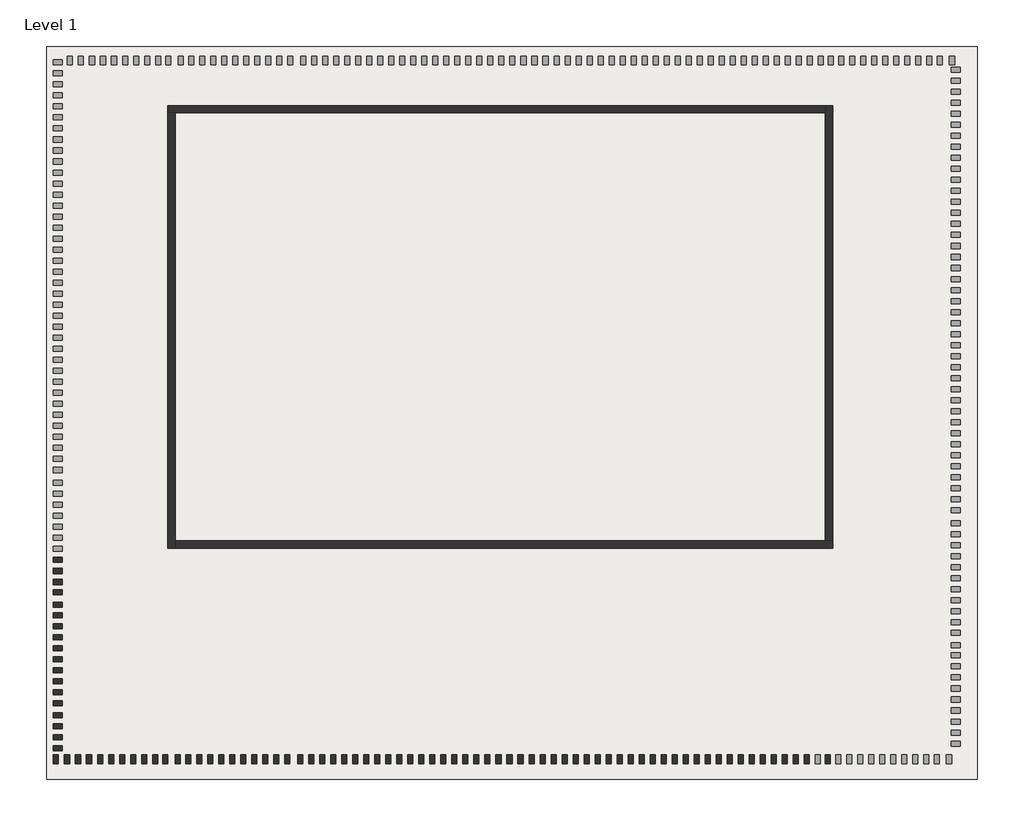
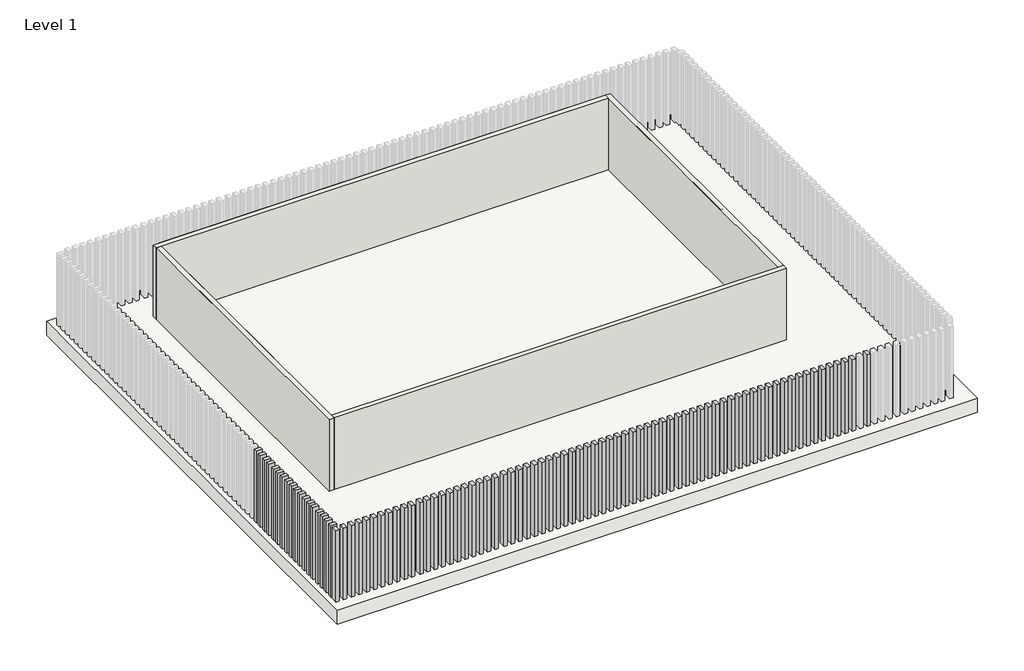
# One storey, part 1 of 3: 88 columns, 7 walls, 1 slab.
"""IFC4 building model written with IfcOpenShell, lengths in millimetres."""

from ifc_helpers import new_model, si_unit, frame, origin, origin_with_axes, place, context, project, spatial, polyline, outline, extrude, faceted_brep, transform, mapped, element, save
from components import wood_timber_column_6_x_10_8585acab

model = new_model("IFC4")

# Units and contexts
model_context = context("Model", 3, world=origin())
ifc_project = project(units=[si_unit("LENGTHUNIT", "METRE", prefix="MILLI")], contexts=[model_context])

# Site, building, storey
site = spatial("IfcSite", under=ifc_project)
building = spatial("IfcBuilding", under=site)
storey = spatial("IfcBuildingStorey", under=building, Name="Level 1", Elevation=0.0)

# Columns
placement = place(None, origin())
wood_timber_column_6_x_10_shape = wood_timber_column_6_x_10_8585acab(model_context)
element("IfcColumn", 1, ObjectType="Wood Timber Column : 6 x 10", at=placement, inside=storey, context=model_context, shape_type="MappedRepresentation", body=[
    mapped(wood_timber_column_6_x_10_shape, transform((2543.6966756, -5612.3567338, 0.0), x_axis=(1.0, 0.0, 0.0), y_axis=(0.0, 1.0, 0.0), z_axis=(0.0, 0.0, 1.0))),
])
element("IfcColumn", 2, ObjectType="Wood Timber Column : 6 x 10", at=placement, inside=storey, context=model_context, shape_type="MappedRepresentation", body=[
    mapped(wood_timber_column_6_x_10_shape, transform((1965.8466756, -5612.3567338, 0.0), x_axis=(1.0, 0.0, 0.0), y_axis=(0.0, 1.0, 0.0), z_axis=(0.0, 0.0, 1.0))),
])
element("IfcColumn", 3, ObjectType="Wood Timber Column : 6 x 10", at=placement, inside=storey, context=model_context, shape_type="MappedRepresentation", body=[
    mapped(wood_timber_column_6_x_10_shape, transform((1661.0466756, -5612.3567338, 0.0), x_axis=(1.0, 0.0, 0.0), y_axis=(0.0, 1.0, 0.0), z_axis=(0.0, 0.0, 1.0))),
])
element("IfcColumn", 4, ObjectType="Wood Timber Column : 6 x 10", at=placement, inside=storey, context=model_context, shape_type="MappedRepresentation", body=[
    mapped(wood_timber_column_6_x_10_shape, transform((1356.2466756, -5612.3567338, 0.0), x_axis=(1.0, 0.0, 0.0), y_axis=(0.0, 1.0, 0.0), z_axis=(0.0, 0.0, 1.0))),
])
element("IfcColumn", 5, ObjectType="Wood Timber Column : 6 x 10", at=placement, inside=storey, context=model_context, shape_type="MappedRepresentation", body=[
    mapped(wood_timber_column_6_x_10_shape, transform((1051.4466756, -5612.3567338, 0.0), x_axis=(1.0, 0.0, 0.0), y_axis=(0.0, 1.0, 0.0), z_axis=(0.0, 0.0, 1.0))),
])
element("IfcColumn", 6, ObjectType="Wood Timber Column : 6 x 10", at=placement, inside=storey, context=model_context, shape_type="MappedRepresentation", body=[
    mapped(wood_timber_column_6_x_10_shape, transform((746.6466756, -5612.3567338, 0.0), x_axis=(1.0, 0.0, 0.0), y_axis=(0.0, 1.0, 0.0), z_axis=(0.0, 0.0, 1.0))),
])
element("IfcColumn", 7, ObjectType="Wood Timber Column : 6 x 10", at=placement, inside=storey, context=model_context, shape_type="MappedRepresentation", body=[
    mapped(wood_timber_column_6_x_10_shape, transform((441.8466756, -5612.3567338, 0.0), x_axis=(1.0, 0.0, 0.0), y_axis=(0.0, 1.0, 0.0), z_axis=(0.0, 0.0, 1.0))),
])
element("IfcColumn", 8, ObjectType="Wood Timber Column : 6 x 10", at=placement, inside=storey, context=model_context, shape_type="MappedRepresentation", body=[
    mapped(wood_timber_column_6_x_10_shape, transform((137.0466756, -5612.3567338, 0.0), x_axis=(1.0, 0.0, 0.0), y_axis=(0.0, 1.0, 0.0), z_axis=(0.0, 0.0, 1.0))),
])
element("IfcColumn", 9, ObjectType="Wood Timber Column : 6 x 10", at=placement, inside=storey, context=model_context, shape_type="MappedRepresentation", body=[
    mapped(wood_timber_column_6_x_10_shape, transform((-167.7533244, -5612.3567338, 0.0), x_axis=(1.0, 0.0, 0.0), y_axis=(0.0, 1.0, 0.0), z_axis=(0.0, 0.0, 1.0))),
])
element("IfcColumn", 10, ObjectType="Wood Timber Column : 6 x 10", at=placement, inside=storey, context=model_context, shape_type="MappedRepresentation", body=[
    mapped(wood_timber_column_6_x_10_shape, transform((-472.5533244, -5612.3567338, 0.0), x_axis=(1.0, 0.0, 0.0), y_axis=(0.0, 1.0, 0.0), z_axis=(0.0, 0.0, 1.0))),
])
element("IfcColumn", 11, ObjectType="Wood Timber Column : 6 x 10", at=placement, inside=storey, context=model_context, shape_type="MappedRepresentation", body=[
    mapped(wood_timber_column_6_x_10_shape, transform((-777.3533244, -5612.3567338, 0.0), x_axis=(1.0, 0.0, 0.0), y_axis=(0.0, 1.0, 0.0), z_axis=(0.0, 0.0, 1.0))),
])
element("IfcColumn", 12, ObjectType="Wood Timber Column : 6 x 10", at=placement, inside=storey, context=model_context, shape_type="MappedRepresentation", body=[
    mapped(wood_timber_column_6_x_10_shape, transform((-1082.1533244, -5612.3567338, 0.0), x_axis=(1.0, 0.0, 0.0), y_axis=(0.0, 1.0, 0.0), z_axis=(0.0, 0.0, 1.0))),
])
element("IfcColumn", 13, ObjectType="Wood Timber Column : 6 x 10", at=placement, inside=storey, context=model_context, shape_type="MappedRepresentation", body=[
    mapped(wood_timber_column_6_x_10_shape, transform((-1386.9533244, -5612.3567338, 0.0), x_axis=(1.0, 0.0, 0.0), y_axis=(0.0, 1.0, 0.0), z_axis=(0.0, 0.0, 1.0))),
])
element("IfcColumn", 14, ObjectType="Wood Timber Column : 6 x 10", at=placement, inside=storey, context=model_context, shape_type="MappedRepresentation", body=[
    mapped(wood_timber_column_6_x_10_shape, transform((-1691.7533244, -5612.3567338, 0.0), x_axis=(1.0, 0.0, 0.0), y_axis=(0.0, 1.0, 0.0), z_axis=(0.0, 0.0, 1.0))),
])
element("IfcColumn", 15, ObjectType="Wood Timber Column : 6 x 10", at=placement, inside=storey, context=model_context, shape_type="MappedRepresentation", body=[
    mapped(wood_timber_column_6_x_10_shape, transform((-1996.5533244, -5612.3567338, 0.0), x_axis=(1.0, 0.0, 0.0), y_axis=(0.0, 1.0, 0.0), z_axis=(0.0, 0.0, 1.0))),
])
element("IfcColumn", 16, ObjectType="Wood Timber Column : 6 x 10", at=placement, inside=storey, context=model_context, shape_type="MappedRepresentation", body=[
    mapped(wood_timber_column_6_x_10_shape, transform((-2301.3533244, -5612.3567338, 0.0), x_axis=(1.0, 0.0, 0.0), y_axis=(0.0, 1.0, 0.0), z_axis=(0.0, 0.0, 1.0))),
])
element("IfcColumn", 17, ObjectType="Wood Timber Column : 6 x 10", at=placement, inside=storey, context=model_context, shape_type="MappedRepresentation", body=[
    mapped(wood_timber_column_6_x_10_shape, transform((-2606.1533244, -5612.3567338, 0.0), x_axis=(1.0, 0.0, 0.0), y_axis=(0.0, 1.0, 0.0), z_axis=(0.0, 0.0, 1.0))),
])
element("IfcColumn", 18, ObjectType="Wood Timber Column : 6 x 10", at=placement, inside=storey, context=model_context, shape_type="MappedRepresentation", body=[
    mapped(wood_timber_column_6_x_10_shape, transform((-2910.9533244, -5612.3567338, 0.0), x_axis=(1.0, 0.0, 0.0), y_axis=(0.0, 1.0, 0.0), z_axis=(0.0, 0.0, 1.0))),
])
element("IfcColumn", 19, ObjectType="Wood Timber Column : 6 x 10", at=placement, inside=storey, context=model_context, shape_type="MappedRepresentation", body=[
    mapped(wood_timber_column_6_x_10_shape, transform((-3215.7533244, -5612.3567338, 0.0), x_axis=(1.0, 0.0, 0.0), y_axis=(0.0, 1.0, 0.0), z_axis=(0.0, 0.0, 1.0))),
])
element("IfcColumn", 20, ObjectType="Wood Timber Column : 6 x 10", at=placement, inside=storey, context=model_context, shape_type="MappedRepresentation", body=[
    mapped(wood_timber_column_6_x_10_shape, transform((-3520.5533244, -5612.3567338, 0.0), x_axis=(1.0, 0.0, 0.0), y_axis=(0.0, 1.0, 0.0), z_axis=(0.0, 0.0, 1.0))),
])
element("IfcColumn", 21, ObjectType="Wood Timber Column : 6 x 10", at=placement, inside=storey, context=model_context, shape_type="MappedRepresentation", body=[
    mapped(wood_timber_column_6_x_10_shape, transform((-3825.3533244, -5612.3567338, 0.0), x_axis=(1.0, 0.0, 0.0), y_axis=(0.0, 1.0, 0.0), z_axis=(0.0, 0.0, 1.0))),
])
element("IfcColumn", 22, ObjectType="Wood Timber Column : 6 x 10", at=placement, inside=storey, context=model_context, shape_type="MappedRepresentation", body=[
    mapped(wood_timber_column_6_x_10_shape, transform((-4130.1533244, -5612.3567338, 0.0), x_axis=(1.0, 0.0, 0.0), y_axis=(0.0, 1.0, 0.0), z_axis=(0.0, 0.0, 1.0))),
])
element("IfcColumn", 23, ObjectType="Wood Timber Column : 6 x 10", at=placement, inside=storey, context=model_context, shape_type="MappedRepresentation", body=[
    mapped(wood_timber_column_6_x_10_shape, transform((-4434.9533244, -5612.3567338, 0.0), x_axis=(1.0, 0.0, 0.0), y_axis=(0.0, 1.0, 0.0), z_axis=(0.0, 0.0, 1.0))),
])
element("IfcColumn", 24, ObjectType="Wood Timber Column : 6 x 10", at=placement, inside=storey, context=model_context, shape_type="MappedRepresentation", body=[
    mapped(wood_timber_column_6_x_10_shape, transform((-4739.7533244, -5612.3567338, 0.0), x_axis=(1.0, 0.0, 0.0), y_axis=(0.0, 1.0, 0.0), z_axis=(0.0, 0.0, 1.0))),
])
element("IfcColumn", 25, ObjectType="Wood Timber Column : 6 x 10", at=placement, inside=storey, context=model_context, shape_type="MappedRepresentation", body=[
    mapped(wood_timber_column_6_x_10_shape, transform((-5044.5533244, -5612.3567338, 0.0), x_axis=(1.0, 0.0, 0.0), y_axis=(0.0, 1.0, 0.0), z_axis=(0.0, 0.0, 1.0))),
])
element("IfcColumn", 26, ObjectType="Wood Timber Column : 6 x 10", at=placement, inside=storey, context=model_context, shape_type="MappedRepresentation", body=[
    mapped(wood_timber_column_6_x_10_shape, transform((-5349.3533244, -5612.3567338, 0.0), x_axis=(1.0, 0.0, 0.0), y_axis=(0.0, 1.0, 0.0), z_axis=(0.0, 0.0, 1.0))),
])
element("IfcColumn", 27, ObjectType="Wood Timber Column : 6 x 10", at=placement, inside=storey, context=model_context, shape_type="MappedRepresentation", body=[
    mapped(wood_timber_column_6_x_10_shape, transform((-5654.1533244, -5612.3567338, 0.0), x_axis=(1.0, 0.0, 0.0), y_axis=(0.0, 1.0, 0.0), z_axis=(0.0, 0.0, 1.0))),
])
element("IfcColumn", 28, ObjectType="Wood Timber Column : 6 x 10", at=placement, inside=storey, context=model_context, shape_type="MappedRepresentation", body=[
    mapped(wood_timber_column_6_x_10_shape, transform((-5958.9533244, -5612.3567338, 0.0), x_axis=(1.0, 0.0, 0.0), y_axis=(0.0, 1.0, 0.0), z_axis=(0.0, 0.0, 1.0))),
])
element("IfcColumn", 29, ObjectType="Wood Timber Column : 6 x 10", at=placement, inside=storey, context=model_context, shape_type="MappedRepresentation", body=[
    mapped(wood_timber_column_6_x_10_shape, transform((-6263.7533244, -5612.3567338, 0.0), x_axis=(1.0, 0.0, 0.0), y_axis=(0.0, 1.0, 0.0), z_axis=(0.0, 0.0, 1.0))),
])
element("IfcColumn", 30, ObjectType="Wood Timber Column : 6 x 10", at=placement, inside=storey, context=model_context, shape_type="MappedRepresentation", body=[
    mapped(wood_timber_column_6_x_10_shape, transform((-6568.5533244, -5612.3567338, 0.0), x_axis=(1.0, 0.0, 0.0), y_axis=(0.0, 1.0, 0.0), z_axis=(0.0, 0.0, 1.0))),
])
element("IfcColumn", 31, ObjectType="Wood Timber Column : 6 x 10", at=placement, inside=storey, context=model_context, shape_type="MappedRepresentation", body=[
    mapped(wood_timber_column_6_x_10_shape, transform((-6873.3533244, -5612.3567338, 0.0), x_axis=(1.0, 0.0, 0.0), y_axis=(0.0, 1.0, 0.0), z_axis=(0.0, 0.0, 1.0))),
])
element("IfcColumn", 32, ObjectType="Wood Timber Column : 6 x 10", at=placement, inside=storey, context=model_context, shape_type="MappedRepresentation", body=[
    mapped(wood_timber_column_6_x_10_shape, transform((-7178.1533244, -5612.3567338, 0.0), x_axis=(1.0, 0.0, 0.0), y_axis=(0.0, 1.0, 0.0), z_axis=(0.0, 0.0, 1.0))),
])
element("IfcColumn", 33, ObjectType="Wood Timber Column : 6 x 10", at=placement, inside=storey, context=model_context, shape_type="MappedRepresentation", body=[
    mapped(wood_timber_column_6_x_10_shape, transform((-7482.9533244, -5612.3567338, 0.0), x_axis=(1.0, 0.0, 0.0), y_axis=(0.0, 1.0, 0.0), z_axis=(0.0, 0.0, 1.0))),
])
element("IfcColumn", 34, ObjectType="Wood Timber Column : 6 x 10", at=placement, inside=storey, context=model_context, shape_type="MappedRepresentation", body=[
    mapped(wood_timber_column_6_x_10_shape, transform((-7787.7533244, -5612.3567338, 0.0), x_axis=(1.0, 0.0, 0.0), y_axis=(0.0, 1.0, 0.0), z_axis=(0.0, 0.0, 1.0))),
])
element("IfcColumn", 35, ObjectType="Wood Timber Column : 6 x 10", at=placement, inside=storey, context=model_context, shape_type="MappedRepresentation", body=[
    mapped(wood_timber_column_6_x_10_shape, transform((-8092.5533244, -5612.3567338, 0.0), x_axis=(1.0, 0.0, 0.0), y_axis=(0.0, 1.0, 0.0), z_axis=(0.0, 0.0, 1.0))),
])
element("IfcColumn", 36, ObjectType="Wood Timber Column : 6 x 10", at=placement, inside=storey, context=model_context, shape_type="MappedRepresentation", body=[
    mapped(wood_timber_column_6_x_10_shape, transform((-8397.3533244, -5612.3567338, 0.0), x_axis=(1.0, 0.0, 0.0), y_axis=(0.0, 1.0, 0.0), z_axis=(0.0, 0.0, 1.0))),
])
element("IfcColumn", 37, ObjectType="Wood Timber Column : 6 x 10", at=placement, inside=storey, context=model_context, shape_type="MappedRepresentation", body=[
    mapped(wood_timber_column_6_x_10_shape, transform((-8702.1533244, -5612.3567338, 0.0), x_axis=(1.0, 0.0, 0.0), y_axis=(0.0, 1.0, 0.0), z_axis=(0.0, 0.0, 1.0))),
])
element("IfcColumn", 38, ObjectType="Wood Timber Column : 6 x 10", at=placement, inside=storey, context=model_context, shape_type="MappedRepresentation", body=[
    mapped(wood_timber_column_6_x_10_shape, transform((-9006.9533244, -5612.3567338, 0.0), x_axis=(1.0, 0.0, 0.0), y_axis=(0.0, 1.0, 0.0), z_axis=(0.0, 0.0, 1.0))),
])
element("IfcColumn", 39, ObjectType="Wood Timber Column : 6 x 10", at=placement, inside=storey, context=model_context, shape_type="MappedRepresentation", body=[
    mapped(wood_timber_column_6_x_10_shape, transform((-9311.7533244, -5612.3567338, 0.0), x_axis=(1.0, 0.0, 0.0), y_axis=(0.0, 1.0, 0.0), z_axis=(0.0, 0.0, 1.0))),
])
element("IfcColumn", 40, ObjectType="Wood Timber Column : 6 x 10", at=placement, inside=storey, context=model_context, shape_type="MappedRepresentation", body=[
    mapped(wood_timber_column_6_x_10_shape, transform((-9616.5533244, -5612.3567338, 0.0), x_axis=(1.0, 0.0, 0.0), y_axis=(0.0, 1.0, 0.0), z_axis=(0.0, 0.0, 1.0))),
])
element("IfcColumn", 41, ObjectType="Wood Timber Column : 6 x 10", at=placement, inside=storey, context=model_context, shape_type="MappedRepresentation", body=[
    mapped(wood_timber_column_6_x_10_shape, transform((-9921.3533244, -5612.3567338, 0.0), x_axis=(1.0, 0.0, 0.0), y_axis=(0.0, 1.0, 0.0), z_axis=(0.0, 0.0, 1.0))),
])
element("IfcColumn", 42, ObjectType="Wood Timber Column : 6 x 10", at=placement, inside=storey, context=model_context, shape_type="MappedRepresentation", body=[
    mapped(wood_timber_column_6_x_10_shape, transform((-10226.1533244, -5612.3567338, 0.0), x_axis=(1.0, 0.0, 0.0), y_axis=(0.0, 1.0, 0.0), z_axis=(0.0, 0.0, 1.0))),
])
element("IfcColumn", 43, ObjectType="Wood Timber Column : 6 x 10", at=placement, inside=storey, context=model_context, shape_type="MappedRepresentation", body=[
    mapped(wood_timber_column_6_x_10_shape, transform((-10530.9533244, -5612.3567338, 0.0), x_axis=(1.0, 0.0, 0.0), y_axis=(0.0, 1.0, 0.0), z_axis=(0.0, 0.0, 1.0))),
])
element("IfcColumn", 44, ObjectType="Wood Timber Column : 6 x 10", at=placement, inside=storey, context=model_context, shape_type="MappedRepresentation", body=[
    mapped(wood_timber_column_6_x_10_shape, transform((-10835.7533244, -5612.3567338, 0.0), x_axis=(1.0, 0.0, 0.0), y_axis=(0.0, 1.0, 0.0), z_axis=(0.0, 0.0, 1.0))),
])
element("IfcColumn", 45, ObjectType="Wood Timber Column : 6 x 10", at=placement, inside=storey, context=model_context, shape_type="MappedRepresentation", body=[
    mapped(wood_timber_column_6_x_10_shape, transform((-11140.5533244, -5612.3567338, 0.0), x_axis=(1.0, 0.0, 0.0), y_axis=(0.0, 1.0, 0.0), z_axis=(0.0, 0.0, 1.0))),
])
element("IfcColumn", 46, ObjectType="Wood Timber Column : 6 x 10", at=placement, inside=storey, context=model_context, shape_type="MappedRepresentation", body=[
    mapped(wood_timber_column_6_x_10_shape, transform((-11445.3533244, -5612.3567338, 0.0), x_axis=(1.0, 0.0, 0.0), y_axis=(0.0, 1.0, 0.0), z_axis=(0.0, 0.0, 1.0))),
])
element("IfcColumn", 47, ObjectType="Wood Timber Column : 6 x 10", at=placement, inside=storey, context=model_context, shape_type="MappedRepresentation", body=[
    mapped(wood_timber_column_6_x_10_shape, transform((-11750.1533244, -5612.3567338, 0.0), x_axis=(1.0, 0.0, 0.0), y_axis=(0.0, 1.0, 0.0), z_axis=(0.0, 0.0, 1.0))),
])
element("IfcColumn", 48, ObjectType="Wood Timber Column : 6 x 10", at=placement, inside=storey, context=model_context, shape_type="MappedRepresentation", body=[
    mapped(wood_timber_column_6_x_10_shape, transform((-12054.9533244, -5612.3567338, 0.0), x_axis=(1.0, 0.0, 0.0), y_axis=(0.0, 1.0, 0.0), z_axis=(0.0, 0.0, 1.0))),
])
element("IfcColumn", 49, ObjectType="Wood Timber Column : 6 x 10", at=placement, inside=storey, context=model_context, shape_type="MappedRepresentation", body=[
    mapped(wood_timber_column_6_x_10_shape, transform((-12410.5533244, -5612.3567338, 0.0), x_axis=(1.0, 0.0, 0.0), y_axis=(0.0, 1.0, 0.0), z_axis=(0.0, 0.0, 1.0))),
])
element("IfcColumn", 50, ObjectType="Wood Timber Column : 6 x 10", at=placement, inside=storey, context=model_context, shape_type="MappedRepresentation", body=[
    mapped(wood_timber_column_6_x_10_shape, transform((-12715.3533244, -5612.3567338, 0.0), x_axis=(1.0, 0.0, 0.0), y_axis=(0.0, 1.0, 0.0), z_axis=(0.0, 0.0, 1.0))),
])
element("IfcColumn", 51, ObjectType="Wood Timber Column : 6 x 10", at=placement, inside=storey, context=model_context, shape_type="MappedRepresentation", body=[
    mapped(wood_timber_column_6_x_10_shape, transform((-13020.1533244, -5612.3567338, 0.0), x_axis=(1.0, 0.0, 0.0), y_axis=(0.0, 1.0, 0.0), z_axis=(0.0, 0.0, 1.0))),
])
element("IfcColumn", 52, ObjectType="Wood Timber Column : 6 x 10", at=placement, inside=storey, context=model_context, shape_type="MappedRepresentation", body=[
    mapped(wood_timber_column_6_x_10_shape, transform((-13324.9533244, -5612.3567338, 0.0), x_axis=(1.0, 0.0, 0.0), y_axis=(0.0, 1.0, 0.0), z_axis=(0.0, 0.0, 1.0))),
])
element("IfcColumn", 53, ObjectType="Wood Timber Column : 6 x 10", at=placement, inside=storey, context=model_context, shape_type="MappedRepresentation", body=[
    mapped(wood_timber_column_6_x_10_shape, transform((-13629.7533244, -5612.3567338, 0.0), x_axis=(1.0, 0.0, 0.0), y_axis=(0.0, 1.0, 0.0), z_axis=(0.0, 0.0, 1.0))),
])
element("IfcColumn", 54, ObjectType="Wood Timber Column : 6 x 10", at=placement, inside=storey, context=model_context, shape_type="MappedRepresentation", body=[
    mapped(wood_timber_column_6_x_10_shape, transform((-13934.5533244, -5612.3567338, 0.0), x_axis=(1.0, 0.0, 0.0), y_axis=(0.0, 1.0, 0.0), z_axis=(0.0, 0.0, 1.0))),
])
element("IfcColumn", 55, ObjectType="Wood Timber Column : 6 x 10", at=placement, inside=storey, context=model_context, shape_type="MappedRepresentation", body=[
    mapped(wood_timber_column_6_x_10_shape, transform((-14239.3533244, -5612.3567338, 0.0), x_axis=(1.0, 0.0, 0.0), y_axis=(0.0, 1.0, 0.0), z_axis=(0.0, 0.0, 1.0))),
])
element("IfcColumn", 56, ObjectType="Wood Timber Column : 6 x 10", at=placement, inside=storey, context=model_context, shape_type="MappedRepresentation", body=[
    mapped(wood_timber_column_6_x_10_shape, transform((-14544.1533244, -5612.3567338, 0.0), x_axis=(1.0, 0.0, 0.0), y_axis=(0.0, 1.0, 0.0), z_axis=(0.0, 0.0, 1.0))),
])
element("IfcColumn", 57, ObjectType="Wood Timber Column : 6 x 10", at=placement, inside=storey, context=model_context, shape_type="MappedRepresentation", body=[
    mapped(wood_timber_column_6_x_10_shape, transform((-14848.9533244, -5612.3567338, 0.0), x_axis=(1.0, 0.0, 0.0), y_axis=(0.0, 1.0, 0.0), z_axis=(0.0, 0.0, 1.0))),
])
element("IfcColumn", 58, ObjectType="Wood Timber Column : 6 x 10", at=placement, inside=storey, context=model_context, shape_type="MappedRepresentation", body=[
    mapped(wood_timber_column_6_x_10_shape, transform((-15153.7533244, -5612.3567338, 0.0), x_axis=(1.0, 0.0, 0.0), y_axis=(0.0, 1.0, 0.0), z_axis=(0.0, 0.0, 1.0))),
])
element("IfcColumn", 59, ObjectType="Wood Timber Column : 6 x 10", at=placement, inside=storey, context=model_context, shape_type="MappedRepresentation", body=[
    mapped(wood_timber_column_6_x_10_shape, transform((-15439.5033244, -5612.3567338, 0.0), x_axis=(1.0, 0.0, 0.0), y_axis=(0.0, 1.0, 0.0), z_axis=(0.0, 0.0, 1.0))),
])
element("IfcColumn", 60, ObjectType="Wood Timber Column : 6 x 10", at=placement, inside=storey, context=model_context, shape_type="MappedRepresentation", body=[
    mapped(wood_timber_column_6_x_10_shape, transform((-15782.4033244, -5612.3567338, 0.0), x_axis=(1.0, 0.0, 0.0), y_axis=(0.0, 1.0, 0.0), z_axis=(0.0, 0.0, 1.0))),
])
element("IfcColumn", 61, ObjectType="Wood Timber Column : 6 x 10", at=placement, inside=storey, context=model_context, shape_type="MappedRepresentation", body=[
    mapped(wood_timber_column_6_x_10_shape, transform((-16068.1533244, -5612.3567338, 0.0), x_axis=(1.0, 0.0, 0.0), y_axis=(0.0, 1.0, 0.0), z_axis=(0.0, 0.0, 1.0))),
])
element("IfcColumn", 62, ObjectType="Wood Timber Column : 6 x 10", at=placement, inside=storey, context=model_context, shape_type="MappedRepresentation", body=[
    mapped(wood_timber_column_6_x_10_shape, transform((-16372.9533244, -5612.3567338, 0.0), x_axis=(1.0, 0.0, 0.0), y_axis=(0.0, 1.0, 0.0), z_axis=(0.0, 0.0, 1.0))),
])
element("IfcColumn", 63, ObjectType="Wood Timber Column : 6 x 10", at=placement, inside=storey, context=model_context, shape_type="MappedRepresentation", body=[
    mapped(wood_timber_column_6_x_10_shape, transform((-16677.7533244, -5612.3567338, 0.0), x_axis=(1.0, 0.0, 0.0), y_axis=(0.0, 1.0, 0.0), z_axis=(0.0, 0.0, 1.0))),
])
element("IfcColumn", 64, ObjectType="Wood Timber Column : 6 x 10", at=placement, inside=storey, context=model_context, shape_type="MappedRepresentation", body=[
    mapped(wood_timber_column_6_x_10_shape, transform((-16982.5533244, -5612.3567338, 0.0), x_axis=(1.0, 0.0, 0.0), y_axis=(0.0, 1.0, 0.0), z_axis=(0.0, 0.0, 1.0))),
])
element("IfcColumn", 65, ObjectType="Wood Timber Column : 6 x 10", at=placement, inside=storey, context=model_context, shape_type="MappedRepresentation", body=[
    mapped(wood_timber_column_6_x_10_shape, transform((-17287.3533244, -5612.3567338, 0.0), x_axis=(1.0, 0.0, 0.0), y_axis=(0.0, 1.0, 0.0), z_axis=(0.0, 0.0, 1.0))),
])
element("IfcColumn", 66, ObjectType="Wood Timber Column : 6 x 10", at=placement, inside=storey, context=model_context, shape_type="MappedRepresentation", body=[
    mapped(wood_timber_column_6_x_10_shape, transform((-17592.1533244, -5612.3567338, 0.0), x_axis=(1.0, 0.0, 0.0), y_axis=(0.0, 1.0, 0.0), z_axis=(0.0, 0.0, 1.0))),
])
element("IfcColumn", 67, ObjectType="Wood Timber Column : 6 x 10", at=placement, inside=storey, context=model_context, shape_type="MappedRepresentation", body=[
    mapped(wood_timber_column_6_x_10_shape, transform((-17896.9533244, -5612.3567338, 0.0), x_axis=(1.0, 0.0, 0.0), y_axis=(0.0, 1.0, 0.0), z_axis=(0.0, 0.0, 1.0))),
])
element("IfcColumn", 68, ObjectType="Wood Timber Column : 6 x 10", at=placement, inside=storey, context=model_context, shape_type="MappedRepresentation", body=[
    mapped(wood_timber_column_6_x_10_shape, transform((-18201.7533244, -5612.3567338, 0.0), x_axis=(1.0, 0.0, 0.0), y_axis=(0.0, 1.0, 0.0), z_axis=(0.0, 0.0, 1.0))),
])
element("IfcColumn", 69, ObjectType="Wood Timber Column : 6 x 10", at=placement, inside=storey, context=model_context, shape_type="MappedRepresentation", body=[
    mapped(wood_timber_column_6_x_10_shape, transform((-18506.5533244, -5612.3567338, 0.0), x_axis=(1.0, 0.0, 0.0), y_axis=(0.0, 1.0, 0.0), z_axis=(0.0, 0.0, 1.0))),
])
element("IfcColumn", 70, ObjectType="Wood Timber Column : 6 x 10", at=placement, inside=storey, context=model_context, shape_type="MappedRepresentation", body=[
    mapped(wood_timber_column_6_x_10_shape, transform((-18811.3533244, -5612.3567338, 0.0), x_axis=(1.0, 0.0, 0.0), y_axis=(0.0, 1.0, 0.0), z_axis=(0.0, 0.0, 1.0))),
])
element("IfcColumn", 71, ObjectType="Wood Timber Column : 6 x 10", at=placement, inside=storey, context=model_context, shape_type="MappedRepresentation", body=[
    mapped(wood_timber_column_6_x_10_shape, transform((-18760.5533244, -5307.5567338, 0.0), x_axis=(0.0, 1.0000000000000002, 0.0), y_axis=(-1.0000000000000002, 0.0, 0.0), z_axis=(0.0, 0.0, 1.0))),
])
element("IfcColumn", 72, ObjectType="Wood Timber Column : 6 x 10", at=placement, inside=storey, context=model_context, shape_type="MappedRepresentation", body=[
    mapped(wood_timber_column_6_x_10_shape, transform((-18760.5533244, -5002.7567338, 0.0), x_axis=(0.0, 1.0000000000000004, 0.0), y_axis=(-1.0000000000000004, 0.0, 0.0), z_axis=(0.0, 0.0, 1.0))),
])
element("IfcColumn", 73, ObjectType="Wood Timber Column : 6 x 10", at=placement, inside=storey, context=model_context, shape_type="MappedRepresentation", body=[
    mapped(wood_timber_column_6_x_10_shape, transform((-18760.5533244, -4697.9567338, 0.0), x_axis=(0.0, 1.0000000000000002, 0.0), y_axis=(-1.0000000000000002, 0.0, 0.0), z_axis=(0.0, 0.0, 1.0))),
])
element("IfcColumn", 74, ObjectType="Wood Timber Column : 6 x 10", at=placement, inside=storey, context=model_context, shape_type="MappedRepresentation", body=[
    mapped(wood_timber_column_6_x_10_shape, transform((-18760.5533244, -4393.1567338, 0.0), x_axis=(0.0, 1.0000000000000002, 0.0), y_axis=(-1.0000000000000002, 0.0, 0.0), z_axis=(0.0, 0.0, 1.0))),
])
element("IfcColumn", 75, ObjectType="Wood Timber Column : 6 x 10", at=placement, inside=storey, context=model_context, shape_type="MappedRepresentation", body=[
    mapped(wood_timber_column_6_x_10_shape, transform((-18761.0148275, -100.9347034, 0.0), x_axis=(0.0, 1.0, 0.0), y_axis=(-1.0000000000000002, 0.0, 0.0), z_axis=(0.0, 0.0, 1.0000000000000002))),
])
element("IfcColumn", 76, ObjectType="Wood Timber Column : 6 x 10", at=placement, inside=storey, context=model_context, shape_type="MappedRepresentation", body=[
    mapped(wood_timber_column_6_x_10_shape, transform((-18761.0148275, -405.7347034, 0.0), x_axis=(0.0, 1.0, 0.0), y_axis=(-1.0000000000000002, 0.0, 0.0), z_axis=(0.0, 0.0, 1.0000000000000002))),
])
element("IfcColumn", 77, ObjectType="Wood Timber Column : 6 x 10", at=placement, inside=storey, context=model_context, shape_type="MappedRepresentation", body=[
    mapped(wood_timber_column_6_x_10_shape, transform((-18761.0148275, -710.5347034, 0.0), x_axis=(0.0, 1.0, 0.0), y_axis=(-1.0000000000000002, 0.0, 0.0), z_axis=(0.0, 0.0, 1.0000000000000002))),
])
element("IfcColumn", 78, ObjectType="Wood Timber Column : 6 x 10", at=placement, inside=storey, context=model_context, shape_type="MappedRepresentation", body=[
    mapped(wood_timber_column_6_x_10_shape, transform((-18761.0148275, -996.2847034, 0.0), x_axis=(0.0, 1.0, 0.0), y_axis=(-1.0000000000000002, 0.0, 0.0), z_axis=(0.0, 0.0, 1.0000000000000002))),
])
element("IfcColumn", 79, ObjectType="Wood Timber Column : 6 x 10", at=placement, inside=storey, context=model_context, shape_type="MappedRepresentation", body=[
    mapped(wood_timber_column_6_x_10_shape, transform((-18761.0148275, -1339.1847034, 0.0), x_axis=(0.0, 1.0, 0.0), y_axis=(-1.0000000000000002, 0.0, 0.0), z_axis=(0.0, 0.0, 1.0000000000000002))),
])
element("IfcColumn", 80, ObjectType="Wood Timber Column : 6 x 10", at=placement, inside=storey, context=model_context, shape_type="MappedRepresentation", body=[
    mapped(wood_timber_column_6_x_10_shape, transform((-18761.0148275, -1624.9347034, 0.0), x_axis=(0.0, 1.0, 0.0), y_axis=(-1.0000000000000002, 0.0, 0.0), z_axis=(0.0, 0.0, 1.0000000000000002))),
])
element("IfcColumn", 81, ObjectType="Wood Timber Column : 6 x 10", at=placement, inside=storey, context=model_context, shape_type="MappedRepresentation", body=[
    mapped(wood_timber_column_6_x_10_shape, transform((-18761.0148275, -1929.7347034, 0.0), x_axis=(0.0, 1.0, 0.0), y_axis=(-1.0000000000000002, 0.0, 0.0), z_axis=(0.0, 0.0, 1.0000000000000002))),
])
element("IfcColumn", 82, ObjectType="Wood Timber Column : 6 x 10", at=placement, inside=storey, context=model_context, shape_type="MappedRepresentation", body=[
    mapped(wood_timber_column_6_x_10_shape, transform((-18761.0148275, -2234.5347034, 0.0), x_axis=(0.0, 1.0, 0.0), y_axis=(-1.0000000000000002, 0.0, 0.0), z_axis=(0.0, 0.0, 1.0000000000000002))),
])
element("IfcColumn", 83, ObjectType="Wood Timber Column : 6 x 10", at=placement, inside=storey, context=model_context, shape_type="MappedRepresentation", body=[
    mapped(wood_timber_column_6_x_10_shape, transform((-18761.0148275, -2539.3347034, 0.0), x_axis=(0.0, 1.0, 0.0), y_axis=(-1.0000000000000002, 0.0, 0.0), z_axis=(0.0, 0.0, 1.0000000000000002))),
])
element("IfcColumn", 84, ObjectType="Wood Timber Column : 6 x 10", at=placement, inside=storey, context=model_context, shape_type="MappedRepresentation", body=[
    mapped(wood_timber_column_6_x_10_shape, transform((-18761.0148275, -2844.1347034, 0.0), x_axis=(0.0, 1.0, 0.0), y_axis=(-1.0000000000000002, 0.0, 0.0), z_axis=(0.0, 0.0, 1.0000000000000002))),
])
element("IfcColumn", 85, ObjectType="Wood Timber Column : 6 x 10", at=placement, inside=storey, context=model_context, shape_type="MappedRepresentation", body=[
    mapped(wood_timber_column_6_x_10_shape, transform((-18761.0148275, -3148.9347034, 0.0), x_axis=(0.0, 1.0, 0.0), y_axis=(-1.0000000000000002, 0.0, 0.0), z_axis=(0.0, 0.0, 1.0000000000000002))),
])
element("IfcColumn", 86, ObjectType="Wood Timber Column : 6 x 10", at=placement, inside=storey, context=model_context, shape_type="MappedRepresentation", body=[
    mapped(wood_timber_column_6_x_10_shape, transform((-18761.0148275, -3453.7347034, 0.0), x_axis=(0.0, 1.0, 0.0), y_axis=(-1.0000000000000002, 0.0, 0.0), z_axis=(0.0, 0.0, 1.0000000000000002))),
])
element("IfcColumn", 87, ObjectType="Wood Timber Column : 6 x 10", at=placement, inside=storey, context=model_context, shape_type="MappedRepresentation", body=[
    mapped(wood_timber_column_6_x_10_shape, transform((-18761.0148275, -3758.5347034, 0.0), x_axis=(0.0, 1.0, 0.0), y_axis=(-1.0000000000000002, 0.0, 0.0), z_axis=(0.0, 0.0, 1.0000000000000002))),
])
element("IfcColumn", 88, ObjectType="Wood Timber Column : 6 x 10", at=placement, inside=storey, context=model_context, shape_type="MappedRepresentation", body=[
    mapped(wood_timber_column_6_x_10_shape, transform((-18761.0148275, -4063.3347034, 0.0), x_axis=(0.0, 1.0, 0.0), y_axis=(-1.0000000000000002, 0.0, 0.0), z_axis=(0.0, 0.0, 1.0000000000000002))),
])

# Slab
element("IfcSlab", 89, ObjectType="Generic - 3' white", at=placement, inside=storey, context=model_context, shape_type="SweptSolid", body=[
    extrude(outline(polyline([(6683.4351725, 14104.0152966), (6683.4351725, -6165.1847034), (-19072.1648275, -6165.1847034), (-19072.1648275, 14104.0152966), (6683.4351725, 14104.0152966)])), frame((0.0, 0.0, -609.6), z_axis=(0.0, 0.0, 1.0), x_axis=(1.0, 0.0, 0.0)), (0.0, 0.0, 1.0), 609.6),
])

# Walls
element("IfcWall", 90, ObjectType="Generic - 8\"", at=placement, inside=storey, context=model_context, shape_type="SweptSolid", body=[
    extrude(outline(polyline([(2473.8466756, 12269.3792748), (-15509.3533244, 12269.3792748), (-15509.3533244, 12472.5792748), (2473.8466756, 12472.5792748), (2473.8466756, 12269.3792748)])), origin_with_axes(), (0.0, 0.0, 1.0), 3048.0),
])
element("IfcWall", 91, ObjectType="Generic - 8\"", at=placement, inside=storey, context=model_context, shape_type="SweptSolid", body=[
    extrude(outline(polyline([(-15509.3533244, 12269.3792748), (-15509.3533244, 4446.1792748), (-15712.5533244, 4446.1792748), (-15712.5533244, 12269.3792748), (-15509.3533244, 12269.3792748)])), origin_with_axes(), (0.0, 0.0, 1.0), 3048.0),
])
element("IfcWall", 92, ObjectType="Generic - 8\"", at=placement, inside=storey, context=model_context, shape_type="SweptSolid", body=[
    extrude(outline(polyline([(2473.8466756, 4446.1792748), (2473.8466756, 12269.3792748), (2677.0466756, 12269.3792748), (2677.0466756, 4446.1792748), (2473.8466756, 4446.1792748)])), origin_with_axes(), (0.0, 0.0, 1.0), 3048.0),
])
element("IfcWall", 93, ObjectType="Generic - 8\" wood", at=placement, inside=storey, context=model_context, shape_type="Brep", body=[
    faceted_brep([(-15712.5533244, 12269.3792748, 0.0), (-15509.3533244, 12269.3792748, 0.0), (2473.8466756, 12269.3792748, 0.0), (2473.8466756, 12269.3792748, 3048.0), (-15509.3533244, 12269.3792748, 3048.0), (-15712.5533244, 12269.3792748, 3048.0), (-15712.5533244, 12472.5792748, 0.0), (-15712.5533244, 12472.5792748, 3048.0), (2473.8466756, 12472.5792748, 3048.0), (2473.8466756, 12472.5792748, 0.0)], [[[0, 1, 2, 3, 4, 5]], [[6, 7, 8, 9]], [[2, 1, 0, 6, 9]], [[5, 4, 3, 8, 7]], [[0, 5, 7, 6]], [[3, 2, 9, 8]]]),
])
element("IfcWall", 94, ObjectType="Generic - 8\" wood", at=placement, inside=storey, context=model_context, shape_type="Brep", body=[
    faceted_brep([(-15509.3533244, 229.6432662, 0.0), (-15509.3533244, 432.8432662, 0.0), (-15509.3533244, 12269.3792748, 0.0), (-15509.3533244, 12269.3792748, 3048.0), (-15509.3533244, 432.8432662, 3048.0), (-15509.3533244, 229.6432662, 3048.0), (-15712.5533244, 229.6432662, 0.0), (-15712.5533244, 229.6432662, 3048.0), (-15712.5533244, 12269.3792748, 3048.0), (-15712.5533244, 12269.3792748, 0.0)], [[[0, 1, 2, 3, 4, 5]], [[6, 7, 8, 9]], [[2, 1, 0, 6, 9]], [[5, 4, 3, 8, 7]], [[0, 5, 7, 6]], [[3, 2, 9, 8]]]),
])
element("IfcWall", 95, ObjectType="Generic - 8\" wood", at=placement, inside=storey, context=model_context, shape_type="Brep", body=[
    faceted_brep([(2677.0466756, 432.8432662, 0.0), (2473.8466756, 432.8432662, 0.0), (-15509.3533244, 432.8432662, 0.0), (-15509.3533244, 432.8432662, 3048.0), (2473.8466756, 432.8432662, 3048.0), (2677.0466756, 432.8432662, 3048.0), (2677.0466756, 229.6432662, 0.0), (2677.0466756, 229.6432662, 3048.0), (-15509.3533244, 229.6432662, 3048.0), (-15509.3533244, 229.6432662, 0.0)], [[[0, 1, 2, 3, 4, 5]], [[6, 7, 8, 9]], [[2, 1, 0, 6, 9]], [[5, 4, 3, 8, 7]], [[0, 5, 7, 6]], [[3, 2, 9, 8]]]),
])
element("IfcWall", 96, ObjectType="Generic - 8\" wood", at=placement, inside=storey, context=model_context, shape_type="Brep", body=[
    faceted_brep([(2473.8466756, 12472.5792748, 0.0), (2473.8466756, 12269.3792748, 0.0), (2473.8466756, 432.8432662, 0.0), (2473.8466756, 432.8432662, 3048.0), (2473.8466756, 12269.3792748, 3048.0), (2473.8466756, 12472.5792748, 3048.0), (2677.0466756, 12472.5792748, 0.0), (2677.0466756, 12472.5792748, 3048.0), (2677.0466756, 432.8432662, 3048.0), (2677.0466756, 432.8432662, 0.0)], [[[0, 1, 2, 3, 4, 5]], [[6, 7, 8, 9]], [[2, 1, 0, 6, 9]], [[5, 4, 3, 8, 7]], [[0, 5, 7, 6]], [[3, 2, 9, 8]]]),
])

save(model, "model.ifc")

# Revit data of these elements
# Type "Wood Timber Column : 6 x 10"
#   Assembly Code = "B1010200"
#   Depth = 0' - 9 1/2"
#   Width = 0' - 5 1/2"
#   Material = Softwood, Lumber
# Type "Generic - 3' white"
#   Assembly Code = "B1010"
#   Function = 0
#   Layers, outside or top first: 2' - 0" "Tile, Porcelain, 4in" (function 1)
# Type "Generic - 8\""
#   Assembly Code = "B2010"
#   Layers, outside or top first: 0' - 8" no material (function 1)
# Type "Generic - 8\" wood"
#   Assembly Code = "B2010"
#   Layers, outside or top first: 0' - 8" "Cherry" (function 1)
# Elements 1, 2, 3, 4, 5, 6, 7, 8, 9, 10, 11, 12, 13, 14, 15, 16, 17, 18, 19, 20, 21, 22, 23, 24, 25, 26, 27, 28, 29, 30, 31, 32, 33, 34, 35, 36, 37, 38, 39, 40, 41, 42, 43, 44, 45, 46, 47, 48, 49, 50, 51, 52, 53, 54, 55, 56, 57, 58, 59, 60, 61, 62, 63, 64, 65, 66, 67, 68, 69, 70, 71, 72, 73, 74, 75, 76, 77, 78, 79, 80, 81, 82, 83, 84, 85, 86, 87, 88 (IfcColumn, "Wood Timber Column : 6 x 10")
#   Phase Created = New Construction
#   Materials on its faces: "Softwood, Lumber"
# Element 89 (IfcSlab, "Generic - 3' white")
#   Height Offset From Level = 0' - 0"
#   Phase Created = New Construction
#   Materials on its faces: "Tile, Porcelain, 4in"
# Elements 90, 91, 92 (IfcWall, "Generic - 8\"")
#   Top Offset = 0' - 0"
#   Base Offset = 0' - 0"
#   Unconnected Height = 10' - 0"
#   wall height = 10' - 0"
#   Phase Created = New Construction
#   Base Constraint = Level 1
#   Materials on its faces: "Default Wall"
# Elements 93, 94, 95, 96 (IfcWall, "Generic - 8\" wood")
#   Top Offset = 0' - 0"
#   Base Offset = 0' - 0"
#   Unconnected Height = 10' - 0"
#   wall height = 10' - 0"
#   Phase Created = New Construction
#   Base Constraint = Level 1
#   Materials on its faces: "Cherry"
# Materials
#   "Softwood, Lumber": class "Wood", colour RGB 223 192 134, transparency 0, Description = "Pinus Echinata", Cost = 0
#   "Tile, Porcelain, 4in": class "Generic", colour RGB 89 87 158, transparency 0, Description = "Porcelain tile, 4\", white", Cost = 0
#   "Cherry": class "Wood", colour RGB 238 208 179, transparency 0, Description = "Prunus Serotina", Cost = 0
#   "Default Wall": colour RGB 128 128 128, transparency 0
